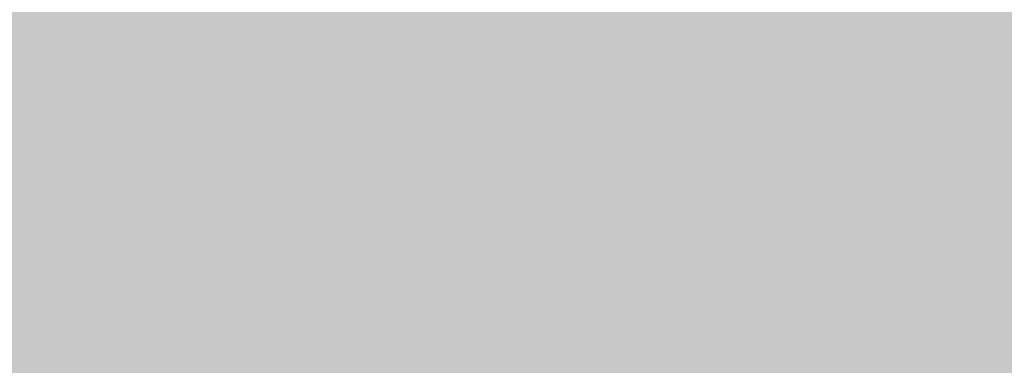
# Model space of a CAD drawing. Units: inches. Extents: x 2091 to 2899, y 967 to 2217.
# Tile 178 of 256: x 2203.151632 to 2203.161218, y 1152.250422 to 1152.253784. Entities that reach past the tile are written whole.
import ezdxf

# ---------------------------------------------------------------- set-up
doc = ezdxf.new("R2010")
doc.units = ezdxf.units.IN
doc.layers.add('A-WALL-PATT', color=141, linetype='Continuous', lineweight=13, true_color=0xadddf7)

msp = doc.modelspace()

# ---------------------------------------------------------------- hatches: boundary and pattern name
at = {"layer": 'A-WALL-PATT'}
h = msp.add_hatch(color=256, dxfattribs=at)
h.dxf.hatch_style = 1
h.paths.add_polyline_path([(2803.1436027, 2050.9190588), (2203.1436027, 2050.9190588), (2203.1436027, 1090.9190588), (2803.1436027, 1090.9190588)])
h.paths.add_polyline_path([(2635.7988501, 1147.5404649), (2674.5240524, 1147.5404649, 0.376086), (2678.5296653, 1152.8802017), (2678.5296653, 1159.5564734, 0.333335), (2674.524319, 1163.561846), (2674.524319, 1163.5618504), (2674.524319, 1192.9343904), (2635.8059707, 1192.9343904), (2597.0876225, 1192.9343904), (2597.0876225, 1163.561846, 0.333335), (2593.0822761, 1159.5564734), (2593.0822761, 1152.8802017, 0.376086), (2597.087889, 1147.5404649)], flags=0)
h.paths.add_polyline_path([(2436.0104329, 1278.2407784, 0.000483), (2435.9526433, 1278.215027, -0.001328), (2435.9356253, 1278.1116934, -0.001711), (2436.1164401, 1278.0407583, 0.002185)], flags=0)
h.paths.add_polyline_path([(2794.1436027, 1143.4190588), (2794.1436027, 1347.4190588), (2543.3701706, 1347.4190588), (2543.3701706, 1351.9190588), (2794.1436027, 1351.9190588), (2794.1436027, 1392.7135549), (2793.9473982, 1392.7135549), (2793.9473982, 1473.5368999), (2794.1436027, 1473.5368999), (2794.1436027, 1531.9190588), (2650.1436027, 1531.9190588), (2650.1436027, 1536.4190588), (2794.1436027, 1536.4190588), (2794.1436027, 1692.4190588), (2609.3756095, 1692.4190588), (2609.3756095, 1644.4190588), (2604.8756095, 1644.4190588), (2604.8756095, 1744.9190588), (2609.3756095, 1744.9190588), (2609.3756095, 1696.9190588), (2794.1436027, 1696.9190588), (2794.1436027, 1780.9190588), (2609.6436027, 1780.9190588), (2493.8756095, 1780.9190588), (2493.8756095, 1785.4190588), (2609.6436027, 1785.4190588), (2794.1436027, 1785.4190588), (2794.1436027, 1847.9388214), (2793.9512217, 1847.9388214), (2793.9512217, 1928.7621663), (2794.1436027, 1928.7621663), (2794.1436027, 1941.4190588), (2614.1436027, 1941.4190588), (2614.1436027, 1821.4190588), (2609.6436027, 1821.4190588), (2609.6436027, 1941.4190588), (2392.1436027, 1941.4190588), (2392.1436027, 1819.9190588), (2387.6436027, 1819.9190588), (2387.6436027, 1941.4190588), (2212.1436027, 1941.4190588), (2212.1436027, 1783.9190588), (2392.1436027, 1783.9190588), (2392.1436027, 1780.9190588), (2212.1436027, 1780.9190588), (2212.1436027, 1629.4190588), (2387.6436027, 1629.4190588), (2387.6436027, 1744.9190588), (2392.1436027, 1744.9190588), (2392.1436027, 1627.9190588), (2317.1436027, 1627.9190588), (2317.1436027, 1551.4190588), (2317.1436027, 1536.4190588), (2459.3835909, 1536.4190588), (2459.3835909, 1602.3964802), (2463.8835909, 1602.3964802), (2463.8835909, 1531.9190588), (2456.6436027, 1531.9190588), (2456.6436027, 1529.9190588), (2452.1436027, 1529.9190588), (2452.1436027, 1531.9190588), (2312.6436027, 1531.9190588), (2312.6436027, 1551.4190588), (2306.1436027, 1551.4190588), (2306.1436027, 1555.9190588), (2308.1436027, 1555.9190588), (2308.1436027, 1551.4190588), (2312.6436027, 1551.4190588), (2312.6436027, 1627.9190588), (2212.1436027, 1627.9190588), (2212.1436027, 1555.9190588), (2270.1436027, 1555.9190588), (2270.1436027, 1551.4190588), (2212.1436027, 1551.4190588), (2212.1436027, 1351.9190588), (2272.1436027, 1351.9190588), (2272.1436027, 1347.4190588), (2212.1436027, 1347.4190588), (2212.1436027, 1275.4190588), (2308.1436027, 1275.4190588), (2308.1436027, 1351.9190588), (2452.1436027, 1351.9190588), (2452.1436027, 1493.9190588), (2456.6436027, 1493.9190588), (2456.6436027, 1347.4190588), (2312.6436027, 1347.4190588), (2312.6436027, 1270.9190588), (2212.1436027, 1270.9190588), (2212.1436027, 1099.9190588), (2281.2375229, 1099.9190588), (2282.8710413, 1110.9138034), (2282.0083413, 1116.9966034), (2278.5577413, 1121.4204034), (2268.2056413, 1128.0562034), (2272.0876413, 1128.0562034), (2273.8129413, 1131.9270034), (2279.4203413, 1134.6919034), (2285.0278413, 1135.2449034), (2287.6158413, 1137.4568034), (2288.0471413, 1138.0098034), (2289.3411413, 1140.7747034), (2291.0665413, 1139.6687034), (2292.3605413, 1135.2449034), (2295.3798413, 1136.9038034), (2296.2425413, 1135.7979034), (2297.1052413, 1133.0330034), (2300.1246413, 1138.0098034), (2303.1439413, 1138.0098034), (2304.4379413, 1135.7979034), (2303.1439413, 1133.5860034), (2306.5946413, 1134.6919034), (2307.8887413, 1133.0330034), (2310.9080413, 1135.2449034), (2313.9274413, 1134.1389034), (2315.6268599, 1132.4271023), (2308.3200413, 1117.5496034), (2290.2038413, 1109.8079034), (2288.9098413, 1103.1721034), (2289.2723086, 1099.9190588), (2434.9182274, 1099.9190588), (2431.5932274, 1124.7880588), (2429.9302274, 1169.5530588), (2430.9271848, 1240.5196942), (2435.6589255, 1238.1861258), (2437.1352274, 1196.5540588), (2438.7982274, 1143.9730588), (2442.6782274, 1111.9980588), (2446.5582274, 1099.9190588), (2794.1436027, 1099.9190588), (2794.1436027, 1138.9190588), (2548.0324471, 1138.9190588), (2548.0324471, 1143.4190588), (2548.0324471, 1148.8190588), (2546.6684571, 1148.0315588), (2528.6856919, 1179.1786218, 0.256256), (2512.0324471, 1148.8190588), (2512.0324471, 1143.4190588), (2512.0324471, 1138.9190588), (2507.5324471, 1138.9190588), (2507.5324471, 1143.4190588), (2507.5324471, 1148.8190588, 0.256256), (2490.8792023, 1179.1786218), (2472.8964371, 1148.0315588), (2471.5324471, 1148.8190588), (2471.5324471, 1143.4190588), (2467.0324471, 1143.4190588), (2467.0324471, 1269.9457858, 0.039061), (2460.9099871, 1273.5800588), (2467.0324471, 1273.5800588), (2467.0324471, 1286.3253638, 0.014511), (2465.2161944, 1286.7619052), (2467.0324471, 1287.0525761), (2467.0324471, 1323.4190588), (2471.5324471, 1323.4190588), (2471.5324471, 1148.8190588), (2489.5324471, 1179.9959734), (2490.8964371, 1179.2084734), (2490.8792023, 1179.1786218, -0.256256), (2507.5324471, 1148.8190588), (2507.5324471, 1143.4190588), (2512.0324471, 1143.4190588), (2512.0324471, 1148.8190588, -0.256256), (2528.6856919, 1179.1786218), (2528.6684571, 1179.2084734), (2530.0324471, 1179.9959734), (2548.0324471, 1148.8190588), (2548.0324471, 1143.4190588)], flags=16)
h.paths.add_polyline_path([(2607.7685461, 1200.9450832), (2607.7685461, 1265.0306251), (2597.0876225, 1281.0520106), (2619.7845852, 1281.0520106), (2627.795278, 1337.1268598), (2635.7988501, 1337.1268598), (2643.8166634, 1337.1268598), (2651.8273562, 1281.0520106), (2674.524319, 1281.0520106), (2663.8433953, 1265.0306251), (2663.8433953, 1200.9450832), (2635.8059707, 1200.9450832)], flags=0)
edge = h.paths.add_edge_path(flags=0)
edge.add_ellipse((13303.8962153, 1272.9987247), major_axis=(-10595.3130399, 0.0000005), ratio=0.842303870086, start_angle=0.62823721906, end_angle=0.64655409989, ccw=False)
edge.add_ellipse((2711.7004495, 1156.8526781), major_axis=(2.2197691, 0), ratio=0.84230387, start_angle=111.5352435, end_angle=180.6282372, ccw=False)
edge.add_ellipse((13303.1562922, 1272.9987246), major_axis=(-10593.0263064, 0), ratio=0.842303869544, start_angle=0.52827147182, end_angle=0.64655409706, ccw=False)
edge.add_line((2710.7645961, 1175.3332951), (2710.1299858, 1175.3332951))
edge.add_ellipse((2710.1299858, 1176.5797752), major_axis=(1.4798461, 0), ratio=0.84230387, start_angle=180, end_angle=270, ccw=False)
edge.add_line((2708.6501397, 1176.5797752), (2708.6501397, 1200.7829144))
edge.add_ellipse((2710.1299858, 1200.7829144), major_axis=(1.4798461, 0), ratio=0.84230387, start_angle=90, end_angle=180, ccw=False)
edge.add_line((2710.1299858, 1202.0293944), (2710.4650752, 1202.0293944))
edge.add_ellipse((13303.1562922, 1272.9987246), major_axis=(-10593.0263064, 0), ratio=0.842303869544, start_angle=-0.09022908859, end_angle=0.38386677879, ccw=False)
edge.add_ellipse((2710.1299858, 1290.9270308), major_axis=(-1.4798461, 0), ratio=0.84230387, start_angle=0, end_angle=90, ccw=False)
edge.add_line((2708.6501397, 1290.9270308), (2708.6501397, 1315.13017))
edge.add_ellipse((2710.1299858, 1315.13017), major_axis=(-1.4798461, 0), ratio=0.84230387, start_angle=-90, end_angle=0, ccw=False)
edge.add_line((2710.1299858, 1316.3766501), (2710.7063141, 1316.3766501))
edge.add_ellipse((3238.4017202, 1296.2895655), major_axis=(528.2339998, 0), ratio=0.84230386954, start_angle=176.349572414, end_angle=177.820049686, ccw=False)
edge.add_ellipse((2775.0630432, 1071.4506962), major_axis=(313.3077613, 0), ratio=0.84230386954, start_angle=102.125965552, end_angle=103.780528989, ccw=False)
edge.add_ellipse((2775.0630432, 1078.3056979), major_axis=(-305.3028915, 0), ratio=0.84230386955, start_angle=-79.790461003, end_angle=-77.555372706, ccw=False)
edge.add_ellipse((2695.1417666, 1541.9753825), major_axis=(-250.9602162, 0), ratio=0.84230386954, start_angle=99.256566007, end_angle=102.554932644)
edge.add_line((2741.4103262, 1334.2142554), (2747.1325454, 1337.3784768))
edge.add_ellipse((2747.5386163, 1336.8574776), major_axis=(-0.739923, 0), ratio=0.84230387, start_angle=270, end_angle=307.9331305, ccw=False)
edge.add_ellipse((2747.5386163, 1336.8574776), major_axis=(-0.739923, 0), ratio=0.84230387, start_angle=232.0668695, end_angle=270, ccw=False)
edge.add_line((2747.9446872, 1337.3784768), (2753.6669064, 1334.2142554))
edge.add_ellipse((2799.935466, 1541.9753825), major_axis=(250.9602162, 0), ratio=0.84230386954, start_angle=257.445067356, end_angle=260.743433993)
edge.add_ellipse((2720.0141894, 1078.3056979), major_axis=(305.3028915, 0), ratio=0.84230386954, start_angle=77.555372707, end_angle=79.790461003, ccw=False)
edge.add_ellipse((2720.0141894, 1071.4506962), major_axis=(-313.3077613, 0), ratio=0.84230386954, start_angle=256.219471011, end_angle=257.874034448, ccw=False)
edge.add_ellipse((2256.6755124, 1296.2895655), major_axis=(-528.2339998, 0), ratio=0.84230386954, start_angle=182.179950314, end_angle=183.650427586, ccw=False)
edge.add_line((2784.3709184, 1316.3766501), (2784.9472468, 1316.3766501))
edge.add_ellipse((2784.9472468, 1315.13017), major_axis=(1.4798461, 0), ratio=0.84230387, start_angle=0, end_angle=90, ccw=False)
edge.add_line((2786.4270928, 1315.13017), (2786.4270928, 1290.9270308))
edge.add_ellipse((2784.9472468, 1290.9270308), major_axis=(1.4798461, 0), ratio=0.84230387, start_angle=270, end_angle=360, ccw=False)
edge.add_ellipse((-7808.0790596, 1272.9987246), major_axis=(10593.0263063, 0), ratio=0.842303869544, start_angle=-0.38386677879, end_angle=0.09022908859, ccw=False)
edge.add_line((2784.6121574, 1202.0293944), (2784.9472468, 1202.0293944))
edge.add_ellipse((2784.9472468, 1200.7829144), major_axis=(1.4798461, 0), ratio=0.84230387, start_angle=0, end_angle=90, ccw=False)
edge.add_line((2786.4270928, 1200.7829144), (2786.4270928, 1176.5797752))
edge.add_ellipse((2784.9472468, 1176.5797752), major_axis=(-1.4798461, 0), ratio=0.84230387, start_angle=90, end_angle=180, ccw=False)
edge.add_line((2784.9472468, 1175.3332951), (2784.3126365, 1175.3332951))
edge.add_ellipse((-7808.0790596, 1272.9987246), major_axis=(10593.0263063, 0), ratio=0.842303869544, start_angle=-0.61864319632, end_angle=-0.52827147182, ccw=False)
edge.add_ellipse((2783.3767831, 1156.8526781), major_axis=(-2.2197691, 0), ratio=0.84230387, start_angle=179.3717628, end_angle=248.4647566, ccw=False)
edge.add_ellipse((-7808.8189826, 1272.9987246), major_axis=(-10595.3130398, 0.0000036), ratio=0.842303865762, start_angle=179.3534459226, end_angle=179.37176280343, ccw=False)
edge.add_ellipse((2780.2973026, 1153.500793), major_axis=(-5.2464256, 0), ratio=0.84230387, start_angle=90, end_angle=179.3534459, ccw=False)
edge.add_line((2780.2973026, 1149.0817084), (2714.77993, 1149.0817084))
edge.add_ellipse((2714.77993, 1153.500793), major_axis=(5.2464256, 0), ratio=0.84230387, start_angle=180.6465541, end_angle=270, ccw=False)
edge = h.paths.add_edge_path(flags=0)
edge.add_line((2718.1873674, 1151.0078329), (2718.1873674, 1170.4723638))
edge.add_ellipse((2721.1470595, 1170.4723638), major_axis=(-2.9596921, 0), ratio=0.84230387, start_angle=-90, end_angle=0, ccw=False)
edge.add_line((2721.1470595, 1172.965324), (2773.9301731, 1172.965324))
edge.add_ellipse((2773.9301731, 1170.4723638), major_axis=(-2.9596921, 0), ratio=0.84230387, start_angle=180, end_angle=270, ccw=False)
edge.add_line((2776.8898652, 1170.4723638), (2776.8898652, 1151.0078329))
edge.add_line((2776.8898652, 1151.0078329), (2718.1873674, 1151.0078329))
edge = h.paths.add_edge_path(flags=0)
edge.add_line((2718.1873674, 1180.2341502), (2718.1873674, 1199.0578342))
edge.add_ellipse((2747.5386163, 1320.3986402), major_axis=(147.0179239, 0), ratio=0.84230386954, start_angle=256.40186531, end_angle=283.59813469)
edge.add_line((2776.8898652, 1199.0578342), (2776.8898652, 1180.2341502))
edge.add_ellipse((2747.5386163, 1301.5749562), major_axis=(147.0179239, 0), ratio=0.84230386954, start_angle=256.40186531, end_angle=283.59813469, ccw=False)
edge = h.paths.add_edge_path(flags=0)
edge.add_ellipse((13303.1562922, 1272.9987246), major_axis=(-10591.5464603, 0), ratio=0.842303869555, start_angle=0.05559431352, end_angle=0.37776419393, ccw=False)
edge.add_line((2711.6168595, 1262.7217103), (2715.6674076, 1249.4953957))
edge.add_ellipse((6413.8919626, 1241.691919), major_axis=(-3698.2361592, 0), ratio=0.842303869547, start_angle=-0.120897369, end_angle=0.3640763489)
edge.add_line((2715.7610383, 1218.1924547), (2711.9343065, 1203.167361))
edge = h.paths.add_edge_path(flags=0)
edge.add_line((2718.1873674, 1251.074566), (2716.0024854, 1267.4504351))
edge.add_ellipse((2742.1511746, 1202.1895399), major_axis=(81.7725845, 0), ratio=0.8423038695, start_angle=94.277420963, end_angle=111.834953797, ccw=False)
edge.add_line((2737.0097482, 1270.9306255), (2758.0674844, 1270.9306255))
edge.add_ellipse((2752.926058, 1202.1895399), major_axis=(81.7725845, 0), ratio=0.8423038695, start_angle=68.165046203, end_angle=85.722579037, ccw=False)
edge.add_line((2779.0747472, 1267.4504351), (2776.8898652, 1251.074566))
edge.add_ellipse((2750.3380588, 1187.8853558), major_axis=(79.5796641, 0), ratio=0.8423038695, start_angle=67.208085122, end_angle=85.129930403)
edge.add_line((2756.0346562, 1254.7436557), (2739.0425764, 1254.7436557))
edge.add_ellipse((2744.7391738, 1187.8853558), major_axis=(79.5796641, 0), ratio=0.8423038695, start_angle=94.870069597, end_angle=112.791914878)
edge = h.paths.add_edge_path(flags=0)
edge.add_line((2783.1429261, 1203.167361), (2779.3161943, 1218.1924547))
edge.add_ellipse((-918.81473, 1241.691919), major_axis=(3698.2361592, 0), ratio=0.842303869546, start_angle=-0.3640763489, end_angle=0.120897369)
edge.add_line((2779.409825, 1249.4953957), (2783.4603731, 1262.7217103))
edge.add_ellipse((-7808.0790596, 1272.9987246), major_axis=(-10591.5464603, 0), ratio=0.84230386954, start_angle=179.6222358061, end_angle=179.94440568651, ccw=False)
edge = h.paths.add_edge_path(flags=0)
edge.add_ellipse((2734.2008921, 1286.6904402), major_axis=(-0.3566086, 6.3400775), ratio=0.603833576, start_angle=89.00201428, end_angle=253.65740805, ccw=False)
edge.add_line((2730.3690013, 1286.5418057), (2730.3690013, 1301.3519803))
edge.add_line((2730.3690013, 1301.3519803), (2735.9133107, 1305.2148028))
edge.add_ellipse((2736.3849168, 1304.7345612), major_axis=(0.739923, 0), ratio=0.84230387, start_angle=90, end_angle=134.4802109, ccw=False)
edge.add_line((2736.3849168, 1305.3578013), (2738.0327829, 1305.3578013))
edge.add_line((2738.0327829, 1305.3578013), (2738.0327829, 1307.7079274))
edge.add_ellipse((2794.201642, 1307.7079274), major_axis=(56.168859, 0), ratio=0.8423038695, start_angle=150.5614304, end_angle=180, ccw=False)
edge.add_ellipse((2700.8755906, 1307.7079274), major_axis=(-56.168859, 0), ratio=0.8423038695, start_angle=180, end_angle=209.4385696, ccw=False)
edge.add_line((2757.0444497, 1307.7079274), (2757.0444497, 1305.3578013))
edge.add_line((2757.0444497, 1305.3578013), (2758.6923157, 1305.3578013))
edge.add_ellipse((2758.6923157, 1304.7345612), major_axis=(-0.739923, 0), ratio=0.84230387, start_angle=225.5197891, end_angle=270, ccw=False)
edge.add_line((2759.1639219, 1305.2148028), (2764.7082312, 1301.3519803))
edge.add_line((2764.7082312, 1301.3519803), (2764.7082312, 1286.5418057))
edge.add_ellipse((2760.8763405, 1286.6904402), major_axis=(0.3566086, 6.3400775), ratio=0.603833576, start_angle=106.34259195, end_angle=270.99798572, ccw=False)
edge.add_line((2757.0444497, 1285.7970896), (2757.0444497, 1307.7079274))
edge.add_ellipse((2700.8755906, 1307.7079274), major_axis=(-56.168859, 0), ratio=0.8423038695, start_angle=180, end_angle=209.4385696)
edge.add_ellipse((2794.201642, 1307.7079274), major_axis=(56.168859, 0), ratio=0.8423038695, start_angle=150.5614304, end_angle=180)
edge.add_line((2738.0327829, 1307.7079274), (2738.0327829, 1285.7970896))
h.paths.add_polyline_path([(2417.8122727, 1104.449704), (2413.4922727, 1102.529704), (2410.6122727, 1103.969704), (2409.1722727, 1106.369704), (2407.2522727, 1107.329704), (2406.2922727, 1109.729704), (2405.3322727, 1114.049704), (2405.3322727, 1117.889704), (2406.2922727, 1120.129704), (2407.2522727, 1119.809704), (2408.8483218, 1118.3276585), (2410.1739451, 1119.4241703), (2410.2112727, 1120.405704), (2411.0407305, 1121.4190541), (2410.6992727, 1119.858704), (2410.1739451, 1119.4241703), (2410.0884515, 1117.1761095), (2411.1328361, 1116.2063237), (2413.9722727, 1119.329704), (2416.8522727, 1120.769704), (2416.8697209, 1120.7987842), (2417.0350713, 1119.4051162), (2417.8962134, 1118.1433844), (2418.2922727, 1118.369704), (2419.5444467, 1120.0392692), (2419.3609153, 1118.387487), (2419.0321078, 1119.3561507), (2418.3989394, 1118.5119262), (2419.2522727, 1114.529704), (2418.7940909, 1107.1987949)], flags=0)
h.paths.add_polyline_path([(2508.8701706, 1347.4190588), (2508.3701706, 1347.4190588), (2508.3701706, 1351.9190588), (2508.8701706, 1351.9190588)], flags=0)
h.paths.add_polyline_path([(2473.3701706, 1347.4190588), (2472.3701706, 1347.4190588), (2467.8701706, 1347.4190588), (2467.8701706, 1455.4190588), (2472.3701706, 1455.4190588), (2472.3701706, 1352.4190588), (2473.3701706, 1352.4190588)], flags=0)
h.paths.add_polyline_path([(2352.106244, 1217.4461971), (2349.226244, 1218.8861971), (2347.786244, 1221.2861971), (2345.866244, 1222.2461971), (2344.906244, 1224.6461971), (2343.946244, 1228.9661971), (2343.946244, 1232.8061971), (2344.906244, 1235.0461971), (2345.866244, 1234.7261971), (2347.4622931, 1233.2441515), (2348.7879164, 1234.3406634), (2348.825244, 1235.3221971), (2349.6547018, 1236.3355471), (2349.313244, 1234.7751971), (2348.7879164, 1234.3406634), (2348.7024228, 1232.0926025), (2349.7468074, 1231.1228168), (2352.586244, 1234.2461971), (2355.466244, 1235.6861971), (2355.4836921, 1235.7152773), (2355.6490426, 1234.3216093), (2356.5101846, 1233.0598774), (2356.906244, 1233.2861971), (2358.1584179, 1234.9557623), (2357.9748866, 1233.3039801), (2357.6460791, 1234.2726438), (2357.0129107, 1233.4284193), (2357.866244, 1229.4461971), (2357.4080622, 1222.115288), (2356.426244, 1219.3661971)], flags=0)
h.paths.add_polyline_path([(2348.2967999, 1112.2244204), (2347.0137999, 1112.3104204), (2345.5297999, 1114.1274204), (2345.7317999, 1115.8584204), (2346.8117999, 1116.9824204), (2346.8117999, 1114.6464204), (2345.8667999, 1114.2144204), (2346.8797999, 1114.3004204)], flags=0)
h.paths.add_polyline_path([(2347.0137999, 1110.9264204), (2346.2717999, 1110.4934204), (2346.6097999, 1111.1864204)], flags=0)
h.paths.add_polyline_path([(2345.8667999, 1118.1944204), (2345.5297999, 1117.3294204), (2343.7077999, 1118.0214204), (2344.3827999, 1118.6264204)], flags=0)
h.paths.add_polyline_path([(2346.6767999, 1109.2824204), (2346.0697999, 1108.0714204), (2345.8667999, 1110.0614204)], flags=0)
h.paths.add_polyline_path([(2345.0567999, 1119.7514204), (2343.6397999, 1119.7514204), (2343.9777999, 1121.1354204)], flags=0)
h.paths.add_polyline_path([(2345.2597999, 1116.5504204), (2345.1247999, 1115.8584204), (2344.9217999, 1115.6854204), (2344.7197999, 1116.3774204)], flags=0)
h.paths.add_polyline_path([(2345.6647999, 1112.3104204), (2345.4617999, 1111.5324204), (2344.0447999, 1111.9644204), (2344.6517999, 1112.5704204)], flags=0)
h.paths.add_polyline_path([(2345.1917999, 1113.3494204), (2344.4497999, 1113.8684204), (2344.7197999, 1114.3874204)], flags=0)
h.paths.add_polyline_path([(2344.6517999, 1116.8094204), (2344.1797999, 1115.6854204), (2344.6517999, 1115.3394204), (2343.9097999, 1114.9064204), (2343.0327999, 1115.9444204), (2343.6397999, 1116.4634204)], flags=0)
h.paths.add_polyline_path([(2345.8667999, 1106.6864204), (2344.9897999, 1105.5624204), (2344.5167999, 1106.6004204)], flags=0)
h.paths.add_polyline_path([(2344.8547999, 1110.0614204), (2344.5167999, 1109.2824204), (2344.1127999, 1109.7154204)], flags=0)
h.paths.add_polyline_path([(2344.0447999, 1113.5224204), (2343.4377999, 1113.0894204), (2342.7627999, 1113.9544204)], flags=0)
h.paths.add_polyline_path([(2344.3147999, 1111.0124204), (2342.9647999, 1110.3204204), (2342.9647999, 1111.0994204)], flags=0)
h.paths.add_polyline_path([(2345.1247999, 1104.6974204), (2344.5847999, 1103.7454204), (2344.4497999, 1104.2644204)], flags=0)
h.paths.add_polyline_path([(2342.8297999, 1121.2224204), (2341.7497999, 1120.5304204), (2340.5357999, 1121.0494204), (2340.1307999, 1121.8284204), (2340.6707999, 1122.9524204), (2341.1427999, 1121.8284204), (2341.6147999, 1122.0014204)], flags=0)
h.paths.add_polyline_path([(2342.9647999, 1119.7514204), (2343.0327999, 1118.4534204), (2342.0877999, 1118.0214204), (2342.0197999, 1119.4914204)], flags=0)
h.paths.add_polyline_path([(2342.6947999, 1116.8964204), (2341.9527999, 1116.6364204), (2342.0197999, 1117.3294204)], flags=0)
h.paths.add_polyline_path([(2343.0327999, 1112.2244204), (2342.0197999, 1111.7914204), (2341.5477999, 1112.2244204), (2342.3577999, 1113.3494204)], flags=0)
h.paths.add_polyline_path([(2343.7747999, 1104.4374204), (2342.6277999, 1102.8804204), (2342.6947999, 1104.6104204), (2343.4377999, 1105.1294204)], flags=0)
h.paths.add_polyline_path([(2342.0197999, 1115.0794204), (2340.8057999, 1115.5124204), (2340.9407999, 1116.3774204)], flags=0)
h.paths.add_polyline_path([(2341.4807999, 1120.0974204), (2341.4807999, 1119.4054204), (2341.0757999, 1119.5784204), (2341.1427999, 1120.0974204)], flags=0)
h.paths.add_polyline_path([(2341.8177999, 1114.4734204), (2340.9407999, 1113.0894204), (2340.8057999, 1114.5604204)], flags=0)
h.paths.add_polyline_path([(2341.1427999, 1118.5404204), (2340.9407999, 1116.9824204), (2339.0507999, 1117.6754204), (2339.0507999, 1118.6264204)], flags=0)
h.paths.add_polyline_path([(2342.6947999, 1101.6684204), (2341.9527999, 1101.8414204), (2342.5597999, 1102.3614204)], flags=0)
h.paths.add_polyline_path([(2340.3327999, 1119.6654204), (2338.4437999, 1119.5784204), (2337.9037999, 1120.3574204), (2339.6577999, 1120.6164204)], flags=0)
h.paths.add_polyline_path([(2340.3327999, 1115.3394204), (2340.0627999, 1113.6954204), (2339.3877999, 1115.3394204)], flags=0)
h.paths.add_polyline_path([(2341.8177999, 1103.8314204), (2341.5477999, 1102.8804204), (2341.1427999, 1103.6584204)], flags=0)
h.paths.add_polyline_path([(2339.0507999, 1122.8664204), (2337.2957999, 1121.8284204), (2337.0937999, 1123.1254204), (2337.7687999, 1123.8184204)], flags=0)
h.paths.add_polyline_path([(2339.1177999, 1121.7414204), (2338.8477999, 1121.2224204), (2338.1737999, 1121.0494204), (2338.3757999, 1121.5684204)], flags=0)
h.paths.add_polyline_path([(2339.1857999, 1119.3194204), (2338.6457999, 1118.7134204), (2338.2407999, 1118.1074204), (2338.2407999, 1118.8864204)], flags=0)
h.paths.add_polyline_path([(2341.1427999, 1101.9284204), (2340.6027999, 1101.2364204), (2340.0627999, 1101.8414204), (2340.6027999, 1102.3614204)], flags=0)
h.paths.add_polyline_path([(2337.6337999, 1117.7614204), (2336.6207999, 1118.2804204), (2337.2957999, 1118.9724204)], flags=0)
h.paths.add_polyline_path([(2336.8237999, 1119.5784204), (2334.7987999, 1118.9724204), (2335.2037999, 1120.3574204), (2336.5537999, 1120.8764204)], flags=0)
h.paths.add_polyline_path([(2339.1177999, 1100.4574204), (2337.3637999, 1100.5434204), (2336.7557999, 1101.2364204)], flags=0)
h.paths.add_polyline_path([(2336.3507999, 1122.4334204), (2336.0137999, 1121.9144204), (2334.9337999, 1122.4334204), (2334.5287999, 1123.4714204), (2335.7437999, 1122.7794204)], flags=0)
h.paths.add_polyline_path([(2334.7317999, 1120.8764204), (2334.2587999, 1120.3574204), (2334.0567999, 1120.7894204), (2334.5967999, 1121.3084204)], flags=0)
h.paths.add_polyline_path([(2334.4617999, 1122.1744204), (2332.5717999, 1121.3084204), (2331.3567999, 1122.1744204), (2332.0997999, 1122.8664204)], flags=0)
h.paths.add_polyline_path([(2334.2587999, 1118.5404204), (2333.3817999, 1118.4534204), (2333.6517999, 1119.3194204)], flags=0)
h.paths.add_polyline_path([(2335.5417999, 1102.2744204), (2334.1917999, 1102.6204204), (2335.2717999, 1103.3124204)], flags=0)
h.paths.add_polyline_path([(2332.7067999, 1119.6654204), (2331.6947999, 1120.4434204), (2332.5047999, 1120.7894204)], flags=0)
h.paths.add_polyline_path([(2334.7317999, 1101.1494204), (2333.5167999, 1101.5824204), (2333.9887999, 1101.7554204)], flags=0)
h.paths.add_polyline_path([(2332.6397999, 1116.6364204), (2331.0867999, 1116.2904204), (2331.9647999, 1118.1944204)], flags=0)
h.paths.add_polyline_path([(2330.7497999, 1121.5684204), (2330.2767999, 1120.2704204), (2328.5227999, 1119.3194204), (2328.9947999, 1121.0494204)], flags=0)
h.paths.add_polyline_path([(2330.7497999, 1118.6264204), (2330.0077999, 1117.5024204), (2329.8727999, 1118.0214204)], flags=0)
h.paths.add_polyline_path([(2332.0997999, 1102.3614204), (2330.5467999, 1102.0144204), (2331.6947999, 1102.9664204)], flags=0)
h.paths.add_polyline_path([(2329.5347999, 1113.6084204), (2329.0627999, 1112.3104204), (2328.5897999, 1113.3494204)], flags=0)
h.paths.add_polyline_path([(2328.3877999, 1117.8484204), (2327.5097999, 1116.5504204), (2327.1727999, 1117.7614204)], flags=0)
h.paths.add_polyline_path([(2329.7377999, 1106.5134204), (2329.5347999, 1105.3024204), (2328.2527999, 1106.0814204)], flags=0)
h.paths.add_polyline_path([(2328.6577999, 1114.3874204), (2328.0497999, 1114.1274204), (2328.3197999, 1114.9064204)], flags=0)
h.paths.add_polyline_path([(2328.3197999, 1112.2244204), (2327.1057999, 1112.1374204), (2326.7007999, 1112.6564204)], flags=0)
h.paths.add_polyline_path([(2326.9027999, 1115.2524204), (2326.7007999, 1114.1274204), (2325.2157999, 1113.6084204), (2326.0927999, 1115.3394204)], flags=0)
h.paths.add_polyline_path([(2326.6327999, 1108.3304204), (2326.0927999, 1107.3794204), (2325.8907999, 1108.5034204), (2326.4977999, 1109.1094204)], flags=0)
h.paths.add_polyline_path([(2615.1436027, 1531.9190588), (2609.6436027, 1531.9190588), (2609.6436027, 1620.4190588), (2614.1436027, 1620.4190588), (2614.1436027, 1536.4190588), (2615.1436027, 1536.4190588)], flags=0)
h.paths.add_polyline_path([(2545.1436027, 1563.4190588), (2464.1436027, 1563.4190588), (2464.1436027, 1632.4190588), (2509.1436027, 1632.4190588), (2509.1436027, 1627.9190588), (2509.1436027, 1603.9190588), (2468.6436027, 1603.9190588), (2468.6436027, 1567.9190588), (2540.6436027, 1567.9190588), (2540.6436027, 1591.9190588), (2545.1436027, 1591.9190588)], flags=0)
h.paths.add_polyline_path([(2388.9690483, 1549.985735), (2357.4341811, 1549.985735), (2357.4341811, 1623.3607783), (2399.3627772, 1623.3607783), (2435.6894654, 1623.3607783), (2435.5925469, 1602.5592734), (2435.5925469, 1602.3964802), (2388.9690483, 1602.3964802)], flags=0)
h.paths.add_polyline_path([(2388.8806282, 1555.8091511), (2374.9044295, 1555.8091511), (2374.9044295, 1600.5715641), (2374.9044295, 1615.4576454), (2406.3508766, 1615.4576454), (2406.3508766, 1618.9394309), (2412.1742927, 1615.4576454), (2406.3508766, 1611.9758599), (2406.3508766, 1615.4576454), (2388.8806282, 1615.4576454)], flags=0)
h.paths.add_polyline_path([(2568.8756095, 1644.4190588), (2453.3756095, 1644.4190588), (2453.3756095, 1785.4190588), (2457.8756095, 1785.4190588), (2457.8756095, 1648.9190588), (2568.8756095, 1648.9190588)], flags=0)
h.paths.add_polyline_path([(2212.1436027, 1945.9190588), (2212.1436027, 2041.9190588), (2794.1436027, 2041.9190588), (2794.1436027, 1945.9190588)], flags=16)
h.paths.add_polyline_path([(2271.0827276, 1964.3172377), (2776.852968, 1964.3172377), (2776.852968, 2037.1696226), (2271.0827276, 2037.1696226)], flags=8)
h.paths.add_polyline_path([(2380.6492852, 1536.8241435), (2461.0408087, 1536.8241435), (2461.0408087, 1554.6525871), (2380.6492852, 1554.6525871)], flags=8)
h.paths.add_polyline_path([(2240.7557092, 1609.7254508), (2309.1858294, 1609.7254508), (2309.1858294, 1617.6982037), (2240.7557092, 1617.6982037)], flags=8)
h.paths.add_polyline_path([(2212.6772554, 1313.5041021), (2282.5915203, 1313.5041021), (2282.5915203, 1322.7452389), (2212.6772554, 1322.7452389)], flags=8)
h.paths.add_polyline_path([(2457.111976, 1114.778574), (2558.4815807, 1114.778574), (2558.4815807, 1142.2196823), (2457.111976, 1142.2196823)], flags=8)
h.paths.add_polyline_path([(2473.4423372, 1273.0100672), (2604.6412257, 1273.0100672), (2604.6412257, 1318.3469349), (2473.4423372, 1318.3469349)], flags=8)
h.paths.add_polyline_path([(2638.8763024, 1626.9774316), (2684.2503675, 1627.9767377), (2684.0384825, 1637.5974944), (2638.6644174, 1636.5981884)], flags=8)
h.paths.add_polyline_path([(2537.5905538, 1453.7934466), (2628.3895472, 1453.7934466), (2628.3895472, 1475.3448114), (2537.5905538, 1475.3448114)], flags=8)
h.paths.add_polyline_path([(2504.1376376, 1714.6323972), (2554.6471875, 1714.6323972), (2554.6471875, 1730.2377115), (2504.1376376, 1730.2377115)], flags=8)
h.paths.add_polyline_path([(2487.5011806, 1575.6518716), (2535.0971214, 1575.6518716), (2535.0971214, 1598.3776456), (2487.5011806, 1598.3776456)], flags=8)
h.paths.add_polyline_path([(2709.0994004, 1735.7102784), (2740.0166009, 1735.7102784), (2740.0166009, 1749.9376406), (2709.0994004, 1749.9376406)], flags=8)
h.paths.add_polyline_path([(2442.4384239, 1792.1716575), (2564.7288353, 1792.1716575), (2564.7288353, 1842.0001626), (2442.4384239, 1842.0001626)], flags=8)
h.paths.add_polyline_path([(2655.8158012, 1809.6440763), (2789.5201425, 1806.6937963), (2790.0849768, 1832.2916379), (2656.3806355, 1835.2419179)], flags=8)
h.paths.add_polyline_path([(2234.8426972, 1797.7201432), (2368.5928512, 1794.7688523), (2369.1607182, 1820.504132), (2235.4105642, 1823.4554229)], flags=8)
h.paths.add_polyline_path([(2245.1384659, 1644.0063348), (2398.4277329, 1640.6238997), (2398.9948417, 1666.3248199), (2245.7055747, 1669.7072549)], flags=8)
h.paths.add_polyline_path([(2306.1428474, 1431.1685186), (2413.7683138, 1428.7936873), (2414.3331481, 1454.3915289), (2306.7076817, 1456.7663602)], flags=8)
h.paths.add_polyline_path([(2306.834582, 1458.2331447), (2393.3804836, 1456.3234487), (2393.9328082, 1481.3543583), (2307.3869066, 1483.2640542)], flags=8)

doc.saveas('drawing.dxf')
